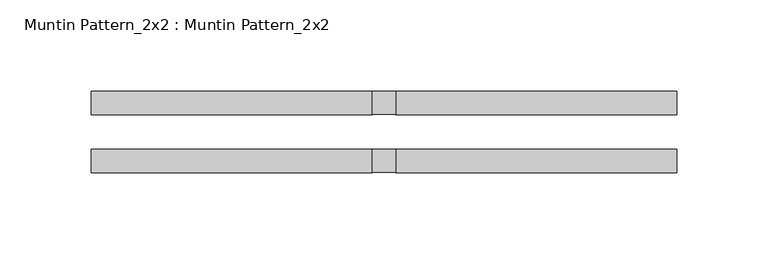
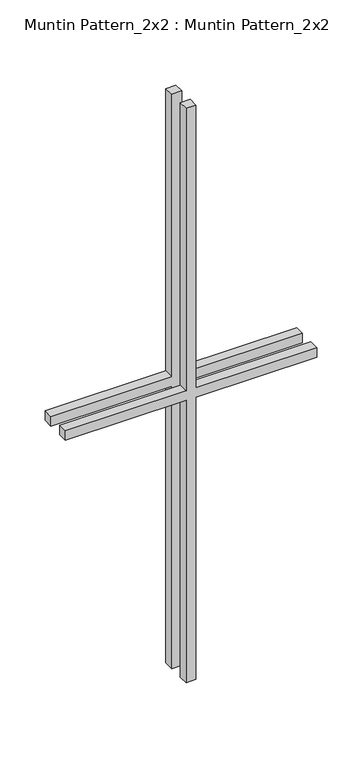
"""IFC4 building model written with IfcOpenShell, lengths in millimetres: proxy geometry, Muntin Pattern_2x2 : Muntin Pattern_2x2."""

from ifc_helpers import new_model, si_unit, frame, origin, place, context, project, spatial, polyline, outline, extrude, source, transform, mapped, element, save


def muntin_pattern_2x2_muntin_pattern_2x2_37b95fb2(model_context):
    return source(origin(), model_context, "Body", "SweptSolid", [
        extrude(outline(polyline([(393.7, -6.35), (393.7, -160.3375), (381.0, -160.3375), (381.0, -6.35), (0.0, -6.35), (0.0, 6.35), (381.0, 6.35), (381.0, 160.3375), (393.7, 160.3375), (393.7, 6.35), (774.7, 6.35), (774.7, -6.35), (393.7, -6.35)])), frame((0.0, -22.225, 0.0), z_axis=(0.0, 1.0, 0.0), x_axis=(0.0, 0.0, 1.0)), (0.0, 0.0, 1.0), 12.7),
        extrude(outline(polyline([(393.7, -6.35), (393.7, -160.3375), (381.0, -160.3375), (381.0, -6.35), (0.0, -6.35), (0.0, 6.35), (381.0, 6.35), (381.0, 160.3375), (393.7, 160.3375), (393.7, 6.35), (774.7, 6.35), (774.7, -6.35), (393.7, -6.35)])), frame((0.0, 9.525, 0.0), z_axis=(0.0, 1.0, 0.0), x_axis=(0.0, 0.0, 1.0)), (0.0, 0.0, 1.0), 12.7),
    ])


if __name__ == "__main__":
    model = new_model("IFC4")
    model_context = context("Model", 3, world=origin())
    ifc_project = project(units=[si_unit("LENGTHUNIT", "METRE", prefix="MILLI")], contexts=[model_context])
    site = spatial("IfcSite", under=ifc_project)
    building = spatial("IfcBuilding", under=site)
    placement = place(None, origin())
    muntin_pattern_2x2_muntin_pattern_2x2_shape = muntin_pattern_2x2_muntin_pattern_2x2_37b95fb2(model_context)
    element("IfcBuildingElementProxy", 1, Name="Muntin Pattern_2x2 : Muntin Pattern_2x2", ObjectType="Muntin Pattern_2x2 : Muntin Pattern_2x2", at=placement, inside=building, context=model_context, shape_type="MappedRepresentation", body=[
        mapped(muntin_pattern_2x2_muntin_pattern_2x2_shape, transform((0.0, 0.0, 0.0), x_axis=(1.0, 0.0, 0.0), y_axis=(0.0, 1.0, 0.0), z_axis=(0.0, 0.0, 1.0))),
    ])
    save(model, "model.ifc")

# Revit data of these elements
# Type "Muntin Pattern_2x2 : Muntin Pattern_2x2"
#   Width [instance default] = 4' - 0"
#   Thickness = 0' - 0 1/2"
#   Height [instance default] = 4' - 0"
#   Distance = 0' - 0 3/4"
#   Interior Material [instance default] = none
#   Exterior Material [instance default] = none
#   Default Elevation = 0
# Element 1 (IfcBuildingElementProxy, "Muntin Pattern_2x2 : Muntin Pattern_2x2")
#   Width = 1' - 0 5/8"
#   Height = 2' - 6 1/2"
#   Interior Material = Wood - Stained
#   Materials on its faces: "Wood - Stained"
# Materials
#   "Wood - Stained": class "Wood", colour RGB 224 178 126, transparency 0, Cost = 0
